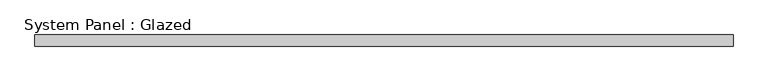
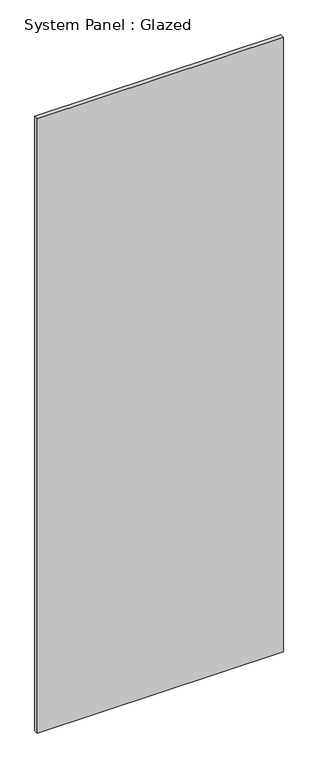
"""IFC4 building model written with IfcOpenShell, lengths in millimetres: plate geometry, System Panel : Glazed."""

from ifc_helpers import new_model, si_unit, origin, origin_with_axes, place, context, project, spatial, polyline, outline, extrude, source, transform, mapped, element, save


def system_panel_glazed_d14c18e3(model_context):
    return source(origin(), model_context, "Body", "SweptSolid", [
        extrude(outline(polyline([(758.4101992, 24.5), (-758.4101992, 24.5), (-758.4101992, 49.5), (758.4101992, 49.5), (758.4101992, 24.5)])), origin_with_axes(), (0.0, 0.0, 1.0), 4000.0),
    ])


if __name__ == "__main__":
    model = new_model("IFC4")
    model_context = context("Model", 3, world=origin())
    ifc_project = project(units=[si_unit("LENGTHUNIT", "METRE", prefix="MILLI")], contexts=[model_context])
    site = spatial("IfcSite", under=ifc_project)
    building = spatial("IfcBuilding", under=site)
    placement = place(None, origin())
    system_panel_glazed_shape = system_panel_glazed_d14c18e3(model_context)
    element("IfcPlate", 1, ObjectType="System Panel : Glazed", at=placement, inside=building, context=model_context, shape_type="MappedRepresentation", body=[
        mapped(system_panel_glazed_shape, transform((0.0, 0.0, 0.0), x_axis=(1.0, 0.0, 0.0), y_axis=(0.0, 1.0, 0.0), z_axis=(0.0, 0.0, 1.0))),
    ])
    save(model, "model.ifc")

# Revit data of these elements
# Type "System Panel : Glazed"
#   Keynote = "H11"
#   Construction Type Id = "GSP4R"
#   Analytic Construction = "1/8 in Pilkington single glazing"
#   Visual Light Transmittance = 0.9
#   Solar Heat Gain Coefficient = 0.86
#   Heat Transfer Coefficient (U) = 6.7069 W/(m²·K)
#   Define Thermal Properties by = 1
# Element 1 (IfcPlate, "System Panel : Glazed")
#   Materials on its faces: "Glass"
# Materials
#   "Glass": class "Glass", colour RGB 0 128 192, transparency 0.9, Description = "Soda Lime Glass", Cost = 0
